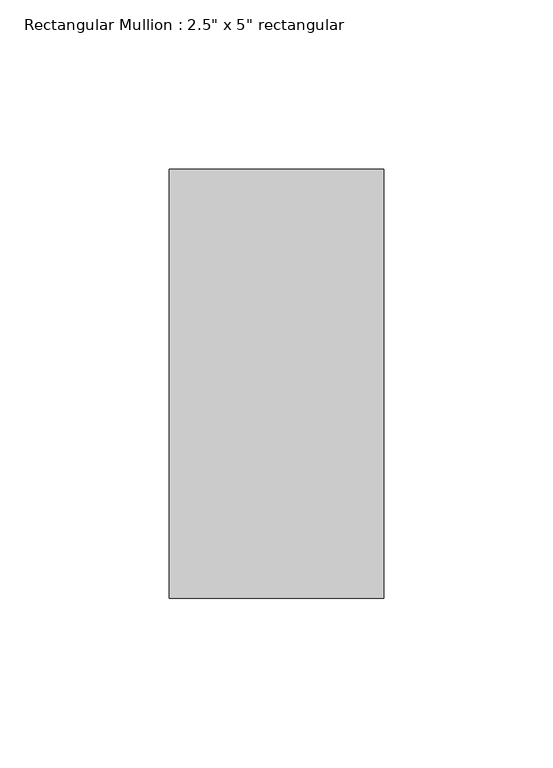
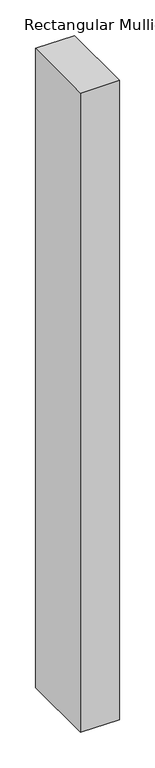
"""IFC4 building model written with IfcOpenShell, lengths in millimetres: member geometry."""

from ifc_helpers import new_model, si_unit, frame, origin, place, context, project, spatial, polyline, outline, extrude, source, transform, mapped, element, save


def member_e80433b6(model_context):
    return source(origin(), model_context, "Body", "SweptSolid", [
        extrude(outline(polyline([(31.75, 63.5), (31.75, -63.5), (-31.75, -63.5), (-31.75, 63.5), (31.75, 63.5)])), frame((0.0, 0.0, -1098.55), z_axis=(0.0, 0.0, 1.0), x_axis=(1.0, 0.0, 0.0)), (0.0, 0.0, 1.0), 1098.55),
    ])


if __name__ == "__main__":
    model = new_model("IFC4")
    model_context = context("Model", 3, world=origin())
    ifc_project = project(units=[si_unit("LENGTHUNIT", "METRE", prefix="MILLI")], contexts=[model_context])
    site = spatial("IfcSite", under=ifc_project)
    building = spatial("IfcBuilding", under=site)
    placement = place(None, origin())
    member_shape = member_e80433b6(model_context)
    element("IfcMember", 1, ObjectType="Rectangular Mullion : 2.5\" x 5\" rectangular", at=placement, inside=building, context=model_context, shape_type="MappedRepresentation", body=[
        mapped(member_shape, transform((0.0, 0.0, 0.0), x_axis=(1.0, 0.0, 0.0), y_axis=(0.0, 1.0, 0.0), z_axis=(0.0, 0.0, 1.0))),
    ])
    save(model, "model.ifc")

# Revit data of these elements
# Type "Rectangular Mullion : 2.5\" x 5\" rectangular"
#   built-in parameter 1007304 = 0.416667 (stored number, unit not read)
#   built-in parameter 1007301 = 0.104167 (stored number, unit not read)
#   built-in parameter 1007300 = 0.104167 (stored number, unit not read)
# Element 1 (IfcMember, "Rectangular Mullion : 2.5\" x 5\" rectangular")
#   Materials on its faces: "Aluminum"
# Materials
#   "Aluminum": class "Metal", colour RGB 247 247 247, transparency 0, Description = "Aluminum 6061", Cost = 0
